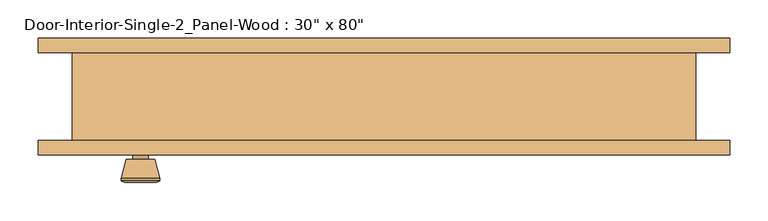
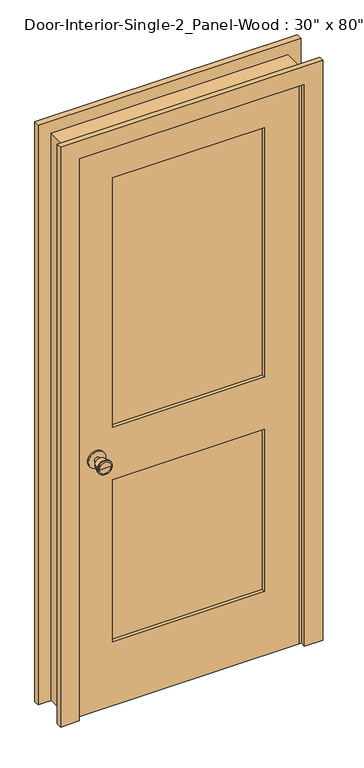
"""IFC4 building model written with IfcOpenShell, lengths in millimetres: door geometry."""

from ifc_helpers import new_model, si_unit, point, frame, frame_2d, origin, place, context, project, spatial, polyline, circle_curve, trimmed, segment, composite_curve, outline, extrude, faceted_brep, source, transform, mapped, element, save
from ifc_brep_helpers import plane_surface, cylinder_surface, revolved_surface, advanced_brep


def door_d6fdea04(model_context):
    return source(origin(), model_context, "Body", "SolidModel", [
        advanced_brep(
        [(-317.5, -13.05, 914.4), (-327.5, -13.05, 914.4), (-307.5, -13.05, 914.4), (-297.0241324, 35.95, 914.4), (-337.9758676, 35.95, 914.4), (-317.5, 35.95, 914.4), (-292.5, 34.1221319, 914.4), (-342.5, 34.1221319, 914.4), (-292.5, 30.6584537, 914.4), (-342.5, 30.6584537, 914.4), (-298.863764, 5.95, 914.4), (-336.136236, 5.95, 914.4), (-307.5, 5.95, 914.4), (-327.5, 5.95, 914.4)],
        [
            (0, 1),
            (1, 2, circle_curve(frame((-317.5, -13.05, 914.4), z_axis=(0.0, -1.0, 0.0), x_axis=(-1.0, 0.0, 0.0)), 10.0)),
            (2, 0),
            (2, 1, circle_curve(frame((-317.5, -13.05, 914.4), z_axis=(0.0, -1.0, 0.0), x_axis=(-1.0, 0.0, 0.0)), 10.0)),
            (3, 4, circle_curve(frame((-317.5, 35.95, 914.4), z_axis=(0.0, 1.0, 0.0), x_axis=(-1.0, 0.0, 0.0)), 20.4758676)),
            (4, 5),
            (5, 3),
            (4, 3, circle_curve(frame((-317.5, 35.95, 914.4), z_axis=(0.0, 1.0, 0.0), x_axis=(-1.0, 0.0, 0.0)), 20.4758676)),
            (6, 7, circle_curve(frame((-317.5, 34.1221319, 914.4), z_axis=(0.0, 1.0, 0.0), x_axis=(-1.0, 0.0, 0.0)), 25.0)),
            (7, 4),
            (3, 6),
            (7, 6, circle_curve(frame((-317.5, 34.1221319, 914.4), z_axis=(0.0, 1.0, 0.0), x_axis=(-1.0, 0.0, 0.0)), 25.0)),
            (8, 9, circle_curve(frame((-317.5, 30.6584537, 914.4), z_axis=(0.0, 1.0, 0.0), x_axis=(-1.0, 0.0, 0.0)), 25.0)),
            (9, 7),
            (6, 8),
            (9, 8, circle_curve(frame((-317.5, 30.6584537, 914.4), z_axis=(0.0, 1.0, 0.0), x_axis=(-1.0, 0.0, 0.0)), 25.0)),
            (10, 11, circle_curve(frame((-317.5, 5.95, 914.4), z_axis=(0.0, 1.0, 0.0), x_axis=(-1.0, 0.0, 0.0)), 18.636236)),
            (11, 9),
            (8, 10),
            (11, 10, circle_curve(frame((-317.5, 5.95, 914.4), z_axis=(0.0, 1.0, 0.0), x_axis=(-1.0, 0.0, 0.0)), 18.636236)),
            (12, 13, circle_curve(frame((-317.5, 5.95, 914.4), z_axis=(0.0, 1.0, 0.0), x_axis=(-1.0, 0.0, 0.0)), 10.0)),
            (13, 11),
            (10, 12),
            (13, 12, circle_curve(frame((-317.5, 5.95, 914.4), z_axis=(0.0, 1.0, 0.0), x_axis=(-1.0, 0.0, 0.0)), 10.0)),
            (1, 13),
            (12, 2),
        ],
        [
            plane_surface(frame((-317.5, -13.05, 914.4), z_axis=(0.0, -1.0, 0.0), x_axis=(-1.0, 0.0, 0.0))),
            plane_surface(frame((-317.5, 35.95, 914.4), z_axis=(0.0, 1.0, 0.0), x_axis=(-1.0, 0.0, 0.0))),
            revolved_surface(polyline([(-337.9758676, 35.95, 914.4), (-342.5, 34.1221319, 914.4)]), (-317.5, -13.05, 914.4), (0.0, -1.0, 0.0)),
            cylinder_surface(frame((-317.5, -13.05, 914.4), z_axis=(0.0, -1.0, 0.0), x_axis=(-1.0, 0.0, 0.0)), 25.0),
            revolved_surface(polyline([(-342.5, 30.6584537, 914.4), (-336.136236, 5.95, 914.4)]), (-317.5, -13.05, 914.4), (0.0, -1.0, 0.0)),
            plane_surface(frame((-317.5, 5.95, 914.4), z_axis=(0.0, -1.0, 0.0), x_axis=(-1.0, 0.0, 0.0))),
            cylinder_surface(frame((-317.5, -13.05, 914.4), z_axis=(0.0, -1.0, 0.0), x_axis=(-1.0, 0.0, 0.0)), 10.0),
        ],
        [
            (0, [[1, 2, 3]]),
            (0, [[-3, 4, -1]]),
            (1, [[5, 6, 7]]),
            (1, [[8, -7, -6]]),
            (2, [[9, 10, -5, 11]]),
            (2, [[12, -11, -8, -10]]),
            (3, [[13, 14, -9, 15]]),
            (3, [[16, -15, -12, -14]]),
            (4, [[17, 18, -13, 19]]),
            (4, [[20, -19, -16, -18]]),
            (5, [[21, 22, -17, 23]]),
            (5, [[24, -23, -20, -22]]),
            (6, [[-2, 25, -21, 26]]),
            (6, [[-4, -26, -24, -25]]),
        ],
    ),
        extrude(outline(composite_curve([segment(trimmed(circle_curve(frame_2d((914.4, -317.5)), 30.0), [point((914.4, -347.5))], [point((914.4, -287.5))], False, "CARTESIAN"), True, "CONTINUOUS"), segment(trimmed(circle_curve(frame_2d((914.4, -317.5)), 30.0), [point((914.4, -287.5))], [point((914.4, -347.5))], False, "CARTESIAN"), True, "CONTINUOUS")], self_intersect=False)), frame((0.0, -19.05, 0.0), z_axis=(0.0, 1.0, 0.0), x_axis=(0.0, 0.0, 1.0)), (0.0, 0.0, 1.0), 6.0),
        advanced_brep(
        [(-317.5, -59.975, 914.4), (-307.5, -59.975, 914.4), (-327.5, -59.975, 914.4), (-297.0241324, -108.975, 914.4), (-317.5, -108.975, 914.4), (-337.9758676, -108.975, 914.4), (-292.5, -107.1471319, 914.4), (-342.5, -107.1471319, 914.4), (-292.5, -103.6834537, 914.4), (-342.5, -103.6834537, 914.4), (-298.863764, -78.975, 914.4), (-336.136236, -78.975, 914.4), (-307.5, -78.975, 914.4), (-327.5, -78.975, 914.4)],
        [
            (0, 1),
            (1, 2, circle_curve(frame((-317.5, -59.975, 914.4), z_axis=(0.0, 1.0, 0.0), x_axis=(-1.0, 0.0, 0.0)), 10.0)),
            (2, 0),
            (2, 1, circle_curve(frame((-317.5, -59.975, 914.4), z_axis=(0.0, 1.0, 0.0), x_axis=(-1.0, 0.0, 0.0)), 10.0)),
            (3, 4),
            (4, 5),
            (5, 3, circle_curve(frame((-317.5, -108.975, 914.4), z_axis=(0.0, -1.0, 0.0), x_axis=(-1.0, 0.0, 0.0)), 20.4758676)),
            (3, 5, circle_curve(frame((-317.5, -108.975, 914.4), z_axis=(0.0, -1.0, 0.0), x_axis=(-1.0, 0.0, 0.0)), 20.4758676)),
            (6, 3),
            (5, 7),
            (7, 6, circle_curve(frame((-317.5, -107.1471319, 914.4), z_axis=(0.0, -1.0, 0.0), x_axis=(-1.0, 0.0, 0.0)), 25.0)),
            (6, 7, circle_curve(frame((-317.5, -107.1471319, 914.4), z_axis=(0.0, -1.0, 0.0), x_axis=(-1.0, 0.0, 0.0)), 25.0)),
            (8, 6),
            (7, 9),
            (9, 8, circle_curve(frame((-317.5, -103.6834537, 914.4), z_axis=(0.0, -1.0, 0.0), x_axis=(-1.0, 0.0, 0.0)), 25.0)),
            (8, 9, circle_curve(frame((-317.5, -103.6834537, 914.4), z_axis=(0.0, -1.0, 0.0), x_axis=(-1.0, 0.0, 0.0)), 25.0)),
            (10, 8),
            (9, 11),
            (11, 10, circle_curve(frame((-317.5, -78.975, 914.4), z_axis=(0.0, -1.0, 0.0), x_axis=(-1.0, 0.0, 0.0)), 18.636236)),
            (10, 11, circle_curve(frame((-317.5, -78.975, 914.4), z_axis=(0.0, -1.0, 0.0), x_axis=(-1.0, 0.0, 0.0)), 18.636236)),
            (12, 10),
            (11, 13),
            (13, 12, circle_curve(frame((-317.5, -78.975, 914.4), z_axis=(0.0, -1.0, 0.0), x_axis=(-1.0, 0.0, 0.0)), 10.0)),
            (12, 13, circle_curve(frame((-317.5, -78.975, 914.4), z_axis=(0.0, -1.0, 0.0), x_axis=(-1.0, 0.0, 0.0)), 10.0)),
            (1, 12),
            (13, 2),
        ],
        [
            plane_surface(frame((-317.5, -59.975, 914.4), z_axis=(0.0, 1.0, 0.0), x_axis=(-1.0, 0.0, 0.0))),
            plane_surface(frame((-317.5, -108.975, 914.4), z_axis=(0.0, -1.0, 0.0), x_axis=(-1.0, 0.0, 0.0))),
            revolved_surface(polyline([(-337.9758676, -108.975, 914.4), (-342.5, -107.1471319, 914.4)]), (-317.5, -59.975, 914.4), (0.0, 1.0, 0.0)),
            cylinder_surface(frame((-317.5, -59.975, 914.4), z_axis=(0.0, 1.0, 0.0), x_axis=(-1.0, 0.0, 0.0)), 25.0),
            revolved_surface(polyline([(-342.5, -103.6834537, 914.4), (-336.136236, -78.975, 914.4)]), (-317.5, -59.975, 914.4), (0.0, 1.0, 0.0)),
            plane_surface(frame((-317.5, -78.975, 914.4), z_axis=(0.0, 1.0, 0.0), x_axis=(-1.0, 0.0, 0.0))),
            cylinder_surface(frame((-317.5, -59.975, 914.4), z_axis=(0.0, 1.0, 0.0), x_axis=(-1.0, 0.0, 0.0)), 10.0),
        ],
        [
            (0, [[1, 2, 3]]),
            (0, [[-3, 4, -1]]),
            (1, [[5, 6, 7]]),
            (1, [[-6, -5, 8]]),
            (2, [[9, -7, 10, 11]]),
            (2, [[-10, -8, -9, 12]]),
            (3, [[13, -11, 14, 15]]),
            (3, [[-14, -12, -13, 16]]),
            (4, [[17, -15, 18, 19]]),
            (4, [[-18, -16, -17, 20]]),
            (5, [[21, -19, 22, 23]]),
            (5, [[-22, -20, -21, 24]]),
            (6, [[25, -23, 26, -2]]),
            (6, [[-26, -24, -25, -4]]),
        ],
    ),
        extrude(outline(composite_curve([segment(trimmed(circle_curve(frame_2d((914.4, -317.5)), 30.0), [point((914.4, -347.5))], [point((914.4, -287.5))], False, "CARTESIAN"), True, "CONTINUOUS"), segment(trimmed(circle_curve(frame_2d((914.4, -317.5)), 30.0), [point((914.4, -287.5))], [point((914.4, -347.5))], False, "CARTESIAN"), True, "CONTINUOUS")], self_intersect=False)), frame((0.0, -59.975, 0.0), z_axis=(0.0, 1.0, 0.0), x_axis=(0.0, 0.0, 1.0)), (0.0, 0.0, 1.0), 6.0),
        faceted_brep([(406.4, -53.975, 0.0), (381.0, -53.975, 0.0), (381.0, -19.05, 0.0), (368.3, -19.05, 0.0), (368.3, 15.875, 0.0), (381.0, 15.875, 0.0), (381.0, 60.325, 0.0), (406.4, 60.325, 0.0), (406.4, 60.325, 2057.4), (406.4, -53.975, 2057.4), (381.0, 60.325, 2032.0), (-381.0, 60.325, 2032.0), (-381.0, 60.325, 0.0), (-406.4, 60.325, 0.0), (-406.4, 60.325, 2057.4), (381.0, 15.875, 2032.0), (368.3, 15.875, 2019.3), (-368.3, 15.875, 2019.3), (-368.3, 15.875, 0.0), (-381.0, 15.875, 0.0), (-381.0, 15.875, 2032.0), (368.3, -19.05, 2019.3), (381.0, -19.05, 2032.0), (-381.0, -19.05, 2032.0), (-381.0, -19.05, 0.0), (-368.3, -19.05, 0.0), (-368.3, -19.05, 2019.3), (381.0, -53.975, 2032.0), (-406.4, -53.975, 2057.4), (-406.4, -53.975, 0.0), (-381.0, -53.975, 0.0), (-381.0, -53.975, 2032.0)], [[[0, 1, 2, 3, 4, 5, 6, 7]], [[7, 8, 9, 0]], [[6, 10, 11, 12, 13, 14, 8, 7]], [[5, 15, 10, 6]], [[4, 16, 17, 18, 19, 20, 15, 5]], [[3, 21, 16, 4]], [[2, 22, 23, 24, 25, 26, 21, 3]], [[1, 27, 22, 2]], [[0, 9, 28, 29, 30, 31, 27, 1]], [[8, 14, 28, 9]], [[15, 20, 11, 10]], [[21, 26, 17, 16]], [[27, 31, 23, 22]], [[29, 13, 12, 19, 18, 25, 24, 30]], [[14, 13, 29, 28]], [[20, 19, 12, 11]], [[26, 25, 18, 17]], [[31, 30, 24, 23]]]),
        extrude(outline(polyline([(2032.0, -381.0), (0.0, -381.0), (0.0, 381.0), (2032.0, 381.0), (2032.0, -381.0)]), holes=[polyline([(1912.9375, -260.35), (1912.9375, 260.35), (1009.65, 260.35), (1009.65, -260.35), (1912.9375, -260.35)]), polyline([(819.15, -260.35), (819.15, 260.35), (231.775, 260.35), (231.775, -260.35), (819.15, -260.35)])]), frame((0.0, -53.975, 0.0), z_axis=(0.0, 1.0, 0.0), x_axis=(0.0, 0.0, 1.0)), (0.0, 0.0, 1.0), 34.925),
        extrude(outline(polyline([(260.35, -30.6916667), (260.35, -42.3333333), (-260.35, -42.3333333), (-260.35, -30.6916667), (260.35, -30.6916667)])), frame((0.0, 0.0, 1009.65), z_axis=(0.0, 0.0, 1.0), x_axis=(1.0, 0.0, 0.0)), (0.0, 0.0, 1.0), 903.2875),
        extrude(outline(polyline([(260.35, -30.6916667), (260.35, -42.3333333), (-260.35, -42.3333333), (-260.35, -30.6916667), (260.35, -30.6916667)])), frame((0.0, 0.0, 231.775), z_axis=(0.0, 0.0, 1.0), x_axis=(1.0, 0.0, 0.0)), (0.0, 0.0, 1.0), 587.375),
        extrude(outline(polyline([(0.0, 450.85), (2101.85, 450.85), (2101.85, -450.85), (0.0, -450.85), (0.0, -387.35), (2038.35, -387.35), (2038.35, 387.35), (0.0, 387.35), (0.0, 450.85)])), frame((0.0, -73.025, 0.0), z_axis=(0.0, 1.0, 0.0), x_axis=(0.0, 0.0, 1.0)), (0.0, 0.0, 1.0), 19.05),
        extrude(outline(polyline([(0.0, 450.85), (2101.85, 450.85), (2101.85, -450.85), (0.0, -450.85), (0.0, -387.35), (2038.35, -387.35), (2038.35, 387.35), (0.0, 387.35), (0.0, 450.85)])), frame((0.0, 60.325, 0.0), z_axis=(0.0, 1.0, 0.0), x_axis=(0.0, 0.0, 1.0)), (0.0, 0.0, 1.0), 19.05),
    ])


if __name__ == "__main__":
    model = new_model("IFC4")
    model_context = context("Model", 3, world=origin())
    ifc_project = project(units=[si_unit("LENGTHUNIT", "METRE", prefix="MILLI")], contexts=[model_context])
    site = spatial("IfcSite", under=ifc_project)
    building = spatial("IfcBuilding", under=site)
    placement = place(None, origin())
    door_shape = door_d6fdea04(model_context)
    element("IfcDoor", 1, ObjectType="Door-Interior-Single-2_Panel-Wood : 30\" x 80\"", at=placement, inside=building, context=model_context, shape_type="MappedRepresentation", body=[
        mapped(door_shape, transform((0.0, 0.0, 0.0), x_axis=(1.0, 0.0, 0.0), y_axis=(0.0, 1.0, 0.0), z_axis=(0.0, 0.0, 1.0))),
    ])
    save(model, "model.ifc")

# Revit data of these elements
# Type "Door-Interior-Single-2_Panel-Wood : 30\" x 80\""
#   Type Mark = "14"
#   Assembly Code = "C1020300"
#   Analytic Construction = "Wooden"
#   Top Rail = 0' - 4 11/16"
#   Thickness = 0' - 1 3/8"
#   Thermal Resistance (R) = 2.5876 (h·ft²·°F)/BTU
#   Swing Angle [instance default] = 90.00°
#   Stiles = 0' - 4 3/4"
#   Rough Width = 2' - 8"
#   Rough Height = 6' - 9"
#   Lock Rail = 0' - 7 1/2"
#   Height = 6' - 8"
#   Width = 2' - 6"
#   Heat Transfer Coefficient (U) = 0.3865 BTU/(h·ft²·°F)
#   Bottom Rail = 0' - 9 1/8"
#   Trim Material = Cherry
#   Panel Material = Cherry
#   Frame Material = Cherry
#   Door Handle Material = Aluminum
#   Visual Light Transmittance = 0
#   Solar Heat Gain Coefficient = 0
#   Wall Closure = (empty or 0)
#   Function = (empty or 0)
# Element 1 (IfcDoor, "Door-Interior-Single-2_Panel-Wood : 30\" x 80\"")
#   Materials on its faces: "Cherry", "Aluminum"
# Materials
#   "Cherry": class "Wood", colour RGB 226 177 128, transparency 0, Description = "Prunus Serotina", Cost = 0
#   "Aluminum": class "Metal", colour RGB 247 247 247, transparency 0, Description = "Aluminum 6061", Cost = 0
